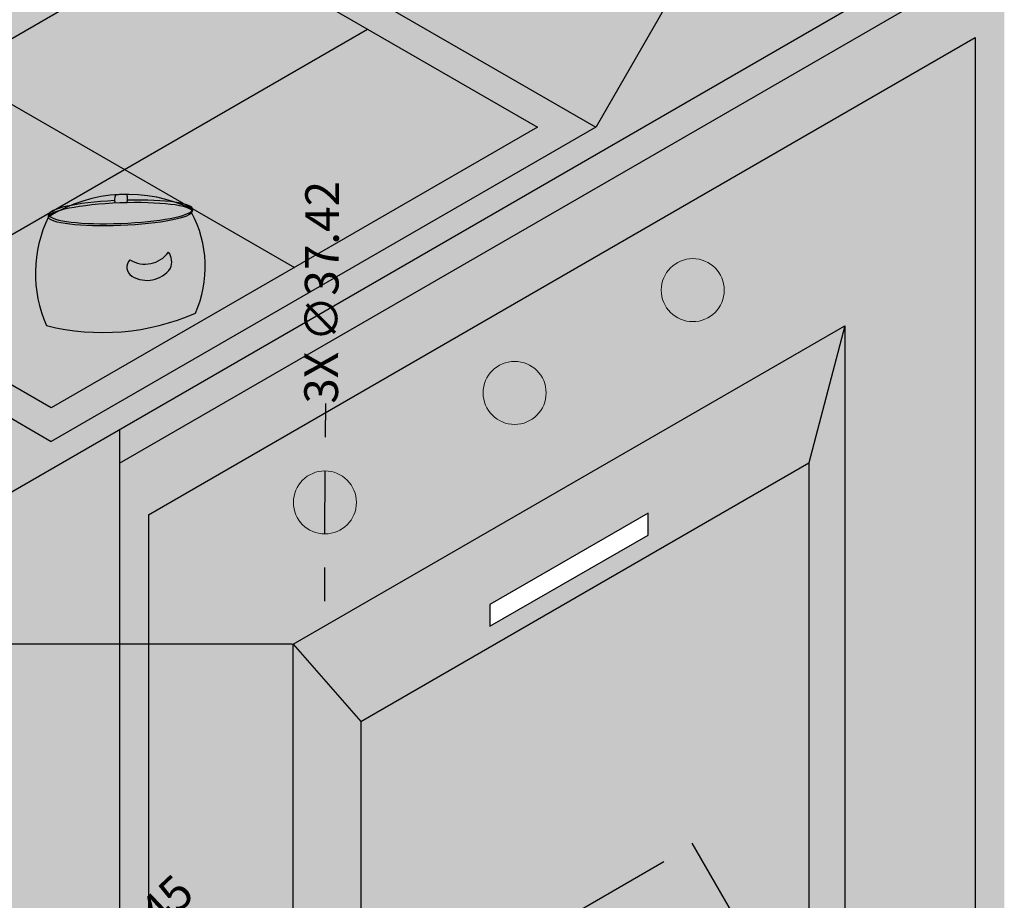
# Model space of a CAD drawing. Units: millimetres. Extents: x 78378 to 86415, y 148682 to 152721.
# Tile 4 of 18: x 79199 to 79783, y 149702 to 150225. Entities that reach past the tile are written whole.
import ezdxf

# ---------------------------------------------------------------- set-up
doc = ezdxf.new("R2010")
doc.units = ezdxf.units.MM
for name, color, linetype, lineweight in [('A-ANNO-DIMS', 2, 'Continuous', 18), ('A-EQPM', 8, 'Continuous', 18), ('A-FURN', 4, 'Continuous', 25), ('A-FURN-PATT', 32, 'Continuous', 13)]:
    doc.layers.add(name, color=color, linetype=linetype, lineweight=lineweight)
doc.styles.get("Standard").update_dxf_attribs({"font": 'arial.ttf'})
doc.dimstyles.new('ISO-25', dxfattribs={"dimtxt": 20, "dimasz": 20, "dimexe": 1.25, "dimexo": 0.625, "dimtad": 0, "dimdec": 1, "dimtxsty": 'Standard', "dimcen": 2.5, "dimadec": 0, "dimazin": 0, "dimtfac": 1, "dimtdec": 1, "dimtmove": 0, "dimatfit": 3, "dimfxl": 1, "dimarcsym": 0})

# ---------------------------------------------------------------- blocks, each defined once
blk = doc.blocks.new('*D22')
at = {"layer": 'A-ANNO-DIMS', "color": 0, "lineweight": -2, "transparency": 16777216}
for p, q in [((80086.091702, 149630.5489088773), (79995.77920202748, 149786.9747473883)), ((79979.08369395178, 149775.8922156335), (79864.48965899751, 149709.7313187051)), ((79710.61581902203, 149620.892215774), (79825.2098539763, 149687.0531127024)), ((79782.98281099998, 149455.5489088774), (79692.67031094636, 149611.9747475287))]:
    blk.add_line(p, q, dxfattribs=at)
at = {"layer": 'A-ANNO-DIMS', "color": 0, "transparency": 16777216}
for points in [[(79977.41702728512, 149778.7789669795), (79980.75036061846, 149773.0054642876), (79996.40420202748, 149785.8922156335)], [(79708.94915235537, 149623.7789671199), (79712.28248568872, 149618.005464428), (79693.29531094636, 149610.892215774)]]:
    blk.add_solid(points, dxfattribs=at)
at = {"layer": 'Defpoints', "color": 0, "transparency": 16777216}
for p in [(79996.40420202748, 149785.8922156335), (80086.404202, 149630.007643), (79783.29531099998, 149455.007643)]:
    blk.add_point(p, dxfattribs=at)
at = {"layer": 'A-ANNO-DIMS', "color": 0, "transparency": 16777216, "insert": (79844.84975648689, 149698.3922157038), "char_height": 20, "attachment_point": 5, "rotation": 30.000000000013433}
blk.add_mtext('350', dxfattribs=at)
blk = doc.blocks.new('*D23')
at = {"layer": 'A-ANNO-DIMS', "color": 0, "lineweight": -2, "transparency": 16777216}
for p, q in [((79304.00747499999, 150298.1287658774), (79213.69497521779, 150454.5546040586)), ((79196.9994671421, 150443.4720723039), (79082.3421139537, 150377.2746185759)), ((78908.23707901475, 150276.7550297867), (79022.8944322031, 150342.9524835145)), ((78980.60407099998, 150111.4117228773), (78890.29157093907, 150267.8375615414))]:
    blk.add_line(p, q, dxfattribs=at)
at = {"layer": 'A-ANNO-DIMS', "color": 0, "transparency": 16777216}
for points in [[(79195.33280047544, 150446.3588236498), (79198.66613380876, 150440.5853209579), (79214.31997521779, 150453.4720723039)], [(78906.57041234808, 150279.6417811326), (78909.90374568143, 150273.8682784407), (78890.91657093907, 150266.7550297866)]]:
    blk.add_solid(points, dxfattribs=at)
at = {"layer": 'Defpoints', "color": 0, "transparency": 16777216}
for p in [(79214.31997521779, 150453.4720723039), (79304.31997499999, 150297.5875), (78980.91657099998, 150110.870457)]:
    blk.add_point(p, dxfattribs=at)
at = {"layer": 'A-ANNO-DIMS', "color": 0, "transparency": 16777216, "insert": (79052.61827307842, 150360.1135510452), "char_height": 20, "attachment_point": 5, "rotation": 30.000000000010683}
blk.add_mtext('373.4', dxfattribs=at)
blk = doc.blocks.new('*D24')
at = {"layer": 'A-ANNO-DIMS', "color": 0, "lineweight": -2, "transparency": 16777216}
for p, q in [((79304.632475, 150298.1287658773), (79394.94497480572, 150454.5546040993)), ((79411.64048288143, 150443.4720723446), (79475.9245159218, 150406.3576685641)), ((79613.47955571176, 150326.9402293129), (79549.19552267138, 150364.0546330934)), ((79541.112564, 150161.5969228774), (79631.42506378744, 150318.0227610676))]:
    blk.add_line(p, q, dxfattribs=at)
at = {"layer": 'A-ANNO-DIMS', "color": 0, "transparency": 16777216}
for points in [[(79413.30714954808, 150446.3588236905), (79409.97381621476, 150440.5853209986), (79394.31997480574, 150453.4720723446)], [(79615.14622237843, 150329.8269806589), (79611.81288904509, 150324.053477967), (79630.80006378744, 150316.9402293129)]]:
    blk.add_solid(points, dxfattribs=at)
at = {"layer": 'Defpoints', "color": 0, "transparency": 16777216}
for p in [(79630.80006378744, 150316.9402293129), (79304.319975, 150297.5874999999), (79540.800064, 150161.055657)]:
    blk.add_point(p, dxfattribs=at)
at = {"layer": 'A-ANNO-DIMS', "color": 0, "transparency": 16777216, "insert": (79512.5600192966, 150385.2061508287), "char_height": 20, "attachment_point": 5, "rotation": 329.9999999999819}
blk.add_mtext('273.06', dxfattribs=at)
blk = doc.blocks.new('*D25')
at = {"layer": 'A-ANNO-DIMS', "color": 0, "lineweight": -2, "transparency": 16777216}
for p, q in [((79360.47687400001, 149854.025187), (78389.60974600006, 149854.025187)), ((78390.85974600006, 149834.025187), (78390.85974600006, 149656.6150549639)), ((78390.85974600006, 149409.864882), (78390.85974600006, 149587.2750140362)), ((79360.47687400001, 149389.8648820001), (78389.60974600006, 149389.8648820001))]:
    blk.add_line(p, q, dxfattribs=at)
at = {"layer": 'A-ANNO-DIMS', "color": 0, "transparency": 16777216}
for points in [[(78387.52641266673, 149834.025187), (78394.19307933339, 149834.025187), (78390.85974600006, 149854.025187)], [(78387.52641266673, 149409.864882), (78394.19307933339, 149409.864882), (78390.85974600006, 149389.8648820001)]]:
    blk.add_solid(points, dxfattribs=at)
at = {"layer": 'Defpoints', "color": 0, "transparency": 16777216}
for p in [(78390.85974600006, 149854.025187), (79361.10187400003, 149854.025187), (79361.10187400003, 149389.8648820001)]:
    blk.add_point(p, dxfattribs=at)
at = {"layer": 'A-ANNO-DIMS', "color": 0, "transparency": 16777216, "insert": (78390.85974600009, 149621.9450345), "char_height": 20, "attachment_point": 5, "rotation": 90}
blk.add_mtext('464.2', dxfattribs=at)
blk = doc.blocks.new('*D26')
at = {"layer": 'A-ANNO-DIMS', "color": 0, "lineweight": -2, "transparency": 16777216}
for p, q in [((79688.22665700002, 149579.4521508773), (79597.91415684896, 149735.8779896975)), ((79581.21864877327, 149724.7954579428), (79462.90800546345, 149656.4887761799)), ((79288.42238213368, 149555.7494545808), (79406.73302544343, 149624.0561363437)), ((79360.78937400001, 149390.4061478773), (79270.47687405797, 149546.8319863355))]:
    blk.add_line(p, q, dxfattribs=at)
at = {"layer": 'A-ANNO-DIMS', "color": 0, "transparency": 16777216}
for points in [[(79579.55198210661, 149727.6822092888), (79582.88531543993, 149721.9087065969), (79598.53915684894, 149734.7954579428)], [(79286.755715467, 149558.6362059267), (79290.08904880035, 149552.8627032348), (79271.10187405799, 149545.7494545808)]]:
    blk.add_solid(points, dxfattribs=at)
at = {"layer": 'Defpoints', "color": 0, "transparency": 16777216}
for p in [(79598.53915684894, 149734.7954579428), (79688.53915700002, 149578.910885), (79361.10187400001, 149389.864882)]:
    blk.add_point(p, dxfattribs=at)
at = {"layer": 'A-ANNO-DIMS', "color": 0, "transparency": 16777216, "insert": (79434.82051545347, 149640.2724562618), "char_height": 20, "attachment_point": 5, "rotation": 29.999999999996074}
blk.add_mtext('378.1', dxfattribs=at)
blk = doc.blocks.new('*D59')
at = {"layer": 'A-ANNO-DIMS', "color": 0, "lineweight": -2, "transparency": 16777216}
for p, q in [((79380.2029535221, 149996.9614811403), (79380.10138026105, 149976.9617390701)), ((79379.809765, 149919.542789), (79379.999807, 149956.961997)), ((79379.70819173894, 149899.5430469298), (79379.60661847789, 149879.5433048597))]:
    blk.add_line(p, q, dxfattribs=at)
at = {"layer": 'A-ANNO-DIMS', "color": 0, "transparency": 16777216}
for points in [[(79376.76808991603, 149976.978667947), (79383.43467060608, 149976.9448101933), (79379.999807, 149956.961997)], [(79376.37490139392, 149899.5599758067), (79383.04148208397, 149899.526118053), (79379.809765, 149919.542789)]]:
    blk.add_solid(points, dxfattribs=at)
at = {"layer": 'Defpoints', "color": 0, "transparency": 16777216}
for p in [(79379.999807, 149956.961997), (79379.809765, 149919.542789)]:
    blk.add_point(p, dxfattribs=at)
at = {"layer": 'A-ANNO-DIMS', "color": 0, "transparency": 16777216, "insert": (79380.53863115159, 150063.0562972237), "char_height": 20, "attachment_point": 5, "rotation": 89.70901279061175}
blk.add_mtext('3X ∅37.42', dxfattribs=at)
blk = doc.blocks.new('*D61')
at = {"layer": 'A-ANNO-DIMS', "color": 0, "lineweight": -2, "transparency": 16777216}
for p, q in [((79224.2464527337, 149639.5853473998), (79209.69247736683, 149625.8674101999)), ((79095.11556299998, 149517.8722489999), (79195.13850199994, 149612.1494729999))]:
    blk.add_line(p, q, dxfattribs=at)
at = {"layer": 'A-ANNO-DIMS', "color": 0, "transparency": 16777216}
blk.add_solid([(79207.40615450018, 149628.293072761), (79211.97880023348, 149623.4417476387), (79195.13850199994, 149612.1494729999)], dxfattribs=at)
at = {"layer": 'Defpoints', "color": 0, "transparency": 16777216}
for p in [(79195.13850199994, 149612.1494729999), (79095.11556299998, 149517.8722489999)]:
    blk.add_point(p, dxfattribs=at)
at = {"layer": 'A-ANNO-DIMS', "color": 0, "transparency": 16777216, "insert": (79261.9300554774, 149675.1042542876), "char_height": 20, "attachment_point": 5, "rotation": 43.30618098475788}
blk.add_mtext('R137.45', dxfattribs=at)

msp = doc.modelspace()

# ---------------------------------------------------------------- hatches: boundary and pattern name
at = {"layer": 'A-FURN-PATT'}
h = msp.add_hatch(color=256, dxfattribs=at)
h.dxf.hatch_style = 1
h.paths.add_polyline_path([(80389.81355980314, 150935.1811176149), (80389.51309381555, 151105.0076434962), (80164.3464888316, 151105.0076434962), (79904.53886769625, 150955.0076434962), (79433.58476952511, 150683.1021681411), (79459.41281351625, 150662.3818050495), (79243.9048024148, 150537.9581968276), (79160.4069246431, 150518.167363956), (78839.3276210414, 150320.0076434962), (78579.51999990609, 150470.0076434961), (78570.85974586825, 150475.0076434961), (78570.85974586825, 150465.0076434962), (78570.85974586825, 149885.0076434961)])
h.paths.add_polyline_path([(80086.40420249099, 150460.0076434961), (79826.59658135568, 150610.0076434961), (78570.85974586825, 149885.0076434961), (78830.66736700358, 149735.0076434961)])
h.paths.add_polyline_path([(79540.80006404899, 150161.0556565937), (79217.39666007676, 149974.3386142535), (78980.9165707482, 150110.8704574853), (79304.31997472048, 150297.5874998256)], flags=16)
h.paths.add_polyline_path([(79506.15904789761, 150161.0556565937), (79217.39666007677, 149994.3386142535), (79015.55758689957, 150110.8704574853), (79304.31997472048, 150277.5874998256)], flags=0)
edge = h.paths.add_edge_path(flags=0)
edge.add_arc((79247.8635885932, 150177.154059363), 137.979927152229, 256.0025927560106, 293.5594108656914)
edge.add_arc((79240.76712928673, 150078.260535577), 68.08549769177299, 336.0991039681863, 387.369687653981)
edge.add_ellipse((79258.3073696606, 150109.4851683714), major_axis=(-42.62344506003415, -1.659142297571932), ratio=0.1604284291443649, start_angle=0, end_angle=179.0977278657225, ccw=False)
edge.add_arc((79285.21118690472, 150074.2509041072), 77.20964330046426, 155.1233103751286, 203.6557939001038)
edge = h.paths.add_edge_path(flags=0)
edge.add_ellipse((79258.69578401413, 150110.8297486024), major_axis=(-42.62344506003415, -1.659142297571932), ratio=0.1604284291443649, start_angle=350.6039411592706, end_angle=356.2289762200799)
edge.add_line((79219.16897707367, 150111.8937051806), (79218.32684768032, 150109.4140931549))
edge.add_arc((79262.46751974897, 150032.9602064517), 88.28134413732826, 112.39312291994881, 119.99999999999571, ccw=False)
h.paths.add_polyline_path([(79287.06250338514, 150086.9702731333, -0.247702064009433), (79288.19674658246, 150077.2955427019, -0.3904765126137986), (79265.47309673205, 150072.5437639662, -0.4872615262363024), (79264.07897218876, 150082.3768585209, 0.3956043262328261)], flags=0)
h.paths.add_polyline_path([(80389.51309381556, 150935.0076434961), (79826.59658135568, 150610.0076434961), (80086.40420249099, 150460.0076434961), (80692.6219851401, 150460.0076434961), (80952.42960627541, 150610.0076434961)])
edge = h.paths.add_edge_path(flags=16)
edge.add_ellipse((80392.44658491029, 150825.6009587087), major_axis=(-133.0756756189512, 7.721978101297283), ratio=0.424499569836956, start_angle=0, end_angle=360)
edge = h.paths.add_edge_path(flags=0)
edge.add_spline(control_points=[(80269.35411604258, 150832.7436415815), (80269.29193278665, 150831.6720147667), (80269.35031475963, 150830.592249842), (80269.73411879689, 150828.3360718096), (80270.06118209881, 150827.1586823489), (80271.04613754865, 150824.6748448987), (80271.70517726007, 150823.3691586005), (80273.40612032128, 150820.6503360826), (80274.44810410585, 150819.2381263036), (80276.93657810257, 150816.3508564802), (80278.3827638828, 150814.8762414973), (80282.58575216534, 150811.0913237019), (80285.62609899955, 150808.7701423959), (80292.60313446997, 150804.2267034199), (80296.53882829295, 150802.0041234762), (80305.19495220963, 150797.7581273222), (80309.91505114386, 150795.7343743789), (80320.0111596611, 150791.9599857595), (80325.38703862559, 150790.2091628441), (80339.21624322617, 150786.3149836253), (80347.95776464436, 150784.3563224224), (80366.06785395242, 150781.2568288573), (80375.43585590576, 150780.1158444778), (80394.309330179, 150778.7158311894), (80403.81420373028, 150778.4568170495), (80422.465596717, 150778.8319300563), (80431.61154730739, 150779.4662025667), (80449.06079653747, 150781.5837654722), (80457.36359407243, 150783.0675039467), (80472.6698529301, 150786.7766095128), (80479.67258750588, 150789.0032721294), (80490.18936031369, 150793.2813222805), (80494.12675567923, 150795.1967122277), (80501.0145611878, 150799.188512515), (80503.9631522054, 150801.2651387212), (80508.20659370373, 150804.9015163823), (80509.7300059309, 150806.4609393726), (80512.19955536906, 150809.4942049083), (80513.14558327098, 150810.9657349426), (80514.42909982229, 150813.5430698013), (80514.84355071915, 150814.6688389962), (80515.39838138374, 150816.8624682529), (80515.5404646545, 150817.9315158847), (80515.58008082317, 150820.0980035506), (80515.47732053277, 150821.197772811), (80514.99049560675, 150823.5061778107), (80514.6046629432, 150824.7154201442), (80513.48543938114, 150827.2641302181), (80512.7510921682, 150828.6026612985), (80510.88722780815, 150831.3808578872), (80509.75776214547, 150832.8196480674), (80507.0873051963, 150835.7513330261), (80505.5466409065, 150837.243857375), (80501.06238832264, 150841.0944478958), (80497.8199298022, 150843.4575549534), (80490.4173793454, 150848.0619874995), (80486.25822277585, 150850.3037143823), (80477.14480578042, 150854.5642972019), (80472.19085006021, 150856.583496544), (80461.6274878137, 150860.3244857693), (80456.01820904585, 150862.0464562905), (80441.73317330678, 150865.8126742317), (80432.78853232553, 150867.6675482482), (80414.33909310326, 150870.5316780972), (80404.8348928345, 150871.5410542788), (80385.7706775062, 150872.6572210053), (80376.21128671143, 150872.7639759942), (80357.54439280283, 150872.0728395342), (80348.43747055416, 150871.27476178), (80331.16822413795, 150868.8299635098), (80323.00642023917, 150867.1826714935), (80309.47200145545, 150863.5363064667), (80303.8627990537, 150861.6592748057), (80293.8018064812, 150857.5400855607), (80289.35122989668, 150855.2968623192), (80282.77569843757, 150851.2345481044), (80280.34726566746, 150849.4578867352), (80276.26060564672, 150845.9127204516), (80274.60404284154, 150844.1457946164), (80272.31573199967, 150841.1242619346), (80271.53575166185, 150839.8453762844), (80270.34961441216, 150837.3878672019), (80269.94168426798, 150836.2101260174), (80269.5065140611, 150834.2814629481), (80269.3988329965, 150833.5142652193), (80269.35411604258, 150832.7436415815)], knot_values=[0, 0, 0, 0, 0.0975004598125087, 0.0975004598125087, 0.1950009196250173, 0.1950009196250173, 0.2925013794375259, 0.2925013794375259, 0.3900018392500346, 0.3900018392500346, 0.4875022990625432, 0.4875022990625432, 0.6388032241337034, 0.6388032241337034, 0.7901041492048636, 0.7901041492048636, 0.9414050742760238, 0.9414050742760238, 1.092705999347184, 1.092705999347184, 1.312817101002443, 1.312817101002443, 1.532928202657702, 1.532928202657702, 1.753039304312961, 1.753039304312961, 1.973150405968221, 1.973150405968221, 2.19326150762348, 2.19326150762348, 2.413372609278739, 2.413372609278739, 2.569860632934037, 2.569860632934037, 2.726348656589336, 2.726348656589336, 2.844186581547077, 2.844186581547077, 2.962024506504818, 2.962024506504818, 3.060233875946405, 3.060233875946405, 3.158443245387991, 3.158443245387991, 3.256652614829578, 3.256652614829578, 3.354861984271164, 3.354861984271164, 3.453071353712751, 3.453071353712751, 3.551280723154337, 3.551280723154337, 3.649490092595923, 3.649490092595923, 3.803927730406353, 3.803927730406353, 3.958365368216782, 3.958365368216782, 4.112803006027212, 4.112803006027212, 4.267240643837642, 4.267240643837642, 4.489203494974081, 4.489203494974081, 4.711166346110521, 4.711166346110521, 4.93312919724696, 4.93312919724696, 5.155092048383399, 5.155092048383399, 5.377054899519838, 5.377054899519838, 5.557853608626545, 5.557853608626545, 5.738652317733252, 5.738652317733252, 5.872395555677483, 5.872395555677483, 6.006138793621714, 6.006138793621714, 6.109604996023907, 6.109604996023907, 6.2130711984261, 6.2130711984261, 6.283185307179586, 6.283185307179586, 6.283185307179586, 6.283185307179586], degree=3, periodic=0)
edge = h.paths.add_edge_path(flags=0)
edge.add_ellipse((80392.446576265, 150825.6009639553), major_axis=(-101.8397670786795, 3.392257208815831), ratio=0.403492477068114, start_angle=0, end_angle=360)
edge = h.paths.add_edge_path(flags=0)
edge.add_ellipse((80391.1657165424, 150858.3745518381), major_axis=(9.088237780547283, -0.67334552975693), ratio=0.3513541290445306, start_angle=0, end_angle=360)
h.paths.add_polyline_path([(80952.42960627541, 150610.0076434961), (80692.62198514014, 150460.0076434962), (81361.23421645904, 150073.9841917607), (81649.96279182703, 150052.7286159431), (81766.49348583283, 150120.0076434961), (81766.49348583283, 150140.0076434961), (81564.90245463562, 150256.396279624), (81564.88840704803, 150096.1962601479), (81538.90760017018, 150111.1962859926), (81538.92165266915, 150271.3963026331)])
h.paths.add_polyline_path([(81539.035680894, 151571.3304684069), (80867.77935513339, 151958.88048878), (80867.77935513337, 151618.8804887802), (81498.02561065964, 151255.0076434964), (81498.02561065964, 150905.0076434961), (81238.21798952435, 150755.0076434961), (81538.94884401507, 150581.3806037023)])
h.paths.add_polyline_path([(81766.49348583283, 151440.0076434962), (81565.01644300755, 151556.3304684069), (81564.92963647815, 150566.38058618), (81766.49348583283, 150450.0076434962)])
edge = h.paths.add_edge_path()
edge.add_line((81564.92963647815, 150566.38058618), (81564.9136990684, 150384.628856009))
edge.add_ellipse((81552.13037602534, 150358.5718270642), major_axis=(52.62721254190076, 3.506026927036754), ratio=0.4958990548584225, start_angle=367.51697565131457, end_angle=420.0564685523974, ccw=False)
edge.add_ellipse((81552.13037602534, 150358.5718270642), major_axis=(52.62721254190076, 3.506026927036754), ratio=0.4958990548584225, start_angle=351.72974196033346, end_angle=367.51697565131457, ccw=False)
edge.add_ellipse((81552.13037602534, 150345.5015529042), major_axis=(52.62721254190076, 3.506026927036754), ratio=0.4958990548584225, start_angle=352.51169489415116, end_angle=366.30060915387577, ccw=False)
edge.add_line((81603.4463374456, 150342.2038825707), (81603.50642755294, 150340.4474978293))
edge.add_ellipse((81552.13037602534, 150332.1280359686), major_axis=(52.62721254190076, 3.506026927036754), ratio=0.4958990548584225, start_angle=353.6729654395227, end_angle=365.38679972494066, ccw=False)
edge.add_ellipse((81552.13037602534, 150332.1280359686), major_axis=(52.62721254190076, 3.506026927036754), ratio=0.4958990548584225, start_angle=350.9388331002564, end_angle=353.6729654395227)
edge.add_line((81603.86882368504, 150329.8549549892), (81604.0441546891, 150324.7301729966))
edge.add_ellipse((81552.13037602534, 150317.7418284518), major_axis=(52.62721254190076, 3.506026927036754), ratio=0.4958990548584225, start_angle=355.21767463173103, end_angle=363.85533637812415, ccw=False)
edge.add_ellipse((81552.13037602534, 150317.7418284518), major_axis=(52.62721254190076, 3.506026927036754), ratio=0.4958990548584225, start_angle=341.3250873036158, end_angle=355.21767463173103, ccw=False)
edge.add_ellipse((81552.13037602534, 150317.7418284518), major_axis=(52.62721254190076, 3.506026927036754), ratio=0.4958990548584225, start_angle=293.4661701367695, end_angle=341.3250873036158, ccw=False)
edge.add_line((81564.90566138821, 150292.9663898651), (81564.90245463562, 150256.396279624))
edge.add_line((81564.90245463562, 150256.396279624), (81766.49348583283, 150140.0076434961))
edge.add_line((81766.49348583283, 150140.0076434961), (81766.49348583283, 150450.0076434962))
edge.add_line((81766.49348583283, 150450.0076434962), (81564.92963647815, 150566.38058618))
h.paths.add_polyline_path([(81525.57129610774, 150321.5980043728), (81526.59848255829, 150321.3069082928), (81528.6771290606, 150320.947049251)])
h.paths.add_polyline_path([(81512.79027333307, 150326.1128631878), (81514.50580755486, 150325.38873887), (81512.53799543541, 150326.2678422534)])
h.paths.add_polyline_path([(81533.21477271736, 150320.1614841748), (81534.69519629495, 150319.9051905676), (81536.59953044976, 150319.755668921)])
h.paths.add_polyline_path([(81518.62200466282, 150323.6512984944), (81519.22704244989, 150323.3959129888), (81521.28902816366, 150322.8115634216)])
h.paths.add_polyline_path([(81501.21834684846, 150336.259909523), (81500.35429342867, 150338.133928838), (81499.78149159584, 150340.0493926212), (81499.50316348342, 150341.9955259773), (81499.50316348343, 150343.7256661642), (81499.75838934928, 150345.5905095656), (81500.27655404429, 150347.4549063508), (81501.05505607055, 150349.3094961287), (81501.09670215519, 150349.3936770376), (81501.13888119749, 150349.4778172982), (81500.99777251929, 150349.749637304), (81500.86282558287, 150350.0225204294), (81499.50316348342, 150355.0658001372), (81499.95910976747, 150359.5002298216), (81501.89819062682, 150363.9082666975), (81505.26528150582, 150368.1645982632), (81509.96466211145, 150372.148224724), (81515.86273756725, 150375.7458987972), (81522.79183627458, 150378.8553451273), (81530.55497651099, 150381.3881677888), (81538.93146626501, 150383.2723632221), (81538.94884401507, 150581.3806037023), (80632.00020687521, 151105.0076434962), (80389.51309381555, 151105.0076434962), (80389.81417426979, 150934.8338146148), (80952.42960627541, 150610.0076434961), (81538.92165266915, 150271.3963026331), (81538.92343538092, 150291.719410528), (81538.87516273293, 150291.7210326448), (81530.1914951021, 150292.8238998863), (81522.18015347481, 150294.6903872688), (81515.08664870211, 150297.2632955209), (81509.86347084012, 150299.9959433281), (81505.6084410237, 150303.1350709547), (81502.41902318504, 150306.608774857), (81500.3682727948, 150310.3374878268), (81499.50316348343, 150314.2358015248), (81499.50316348343, 150315.9659417118), (81499.82059494797, 150318.1159244827), (81500.4869945128, 150320.2634115907), (81501.49791650465, 150322.3940767571), (81500.48699451279, 150324.4232810552), (81499.82059494796, 150326.50388518), (81499.50316348343, 150328.6220090417), (81499.50316348343, 150330.3521492286), (81499.78149159584, 150332.3262168982), (81500.35429342862, 150334.2991697576)])
h = msp.add_hatch(color=256, dxfattribs=at)
h.dxf.hatch_style = 1
h.paths.add_polyline_path([(79783.29531116647, 150265.0076434962), (79783.29531116647, 150285.0076434962), (79257.85559544402, 149981.6448821809), (79257.85559544402, 149961.6448821809)])
h.paths.add_polyline_path([(80086.40420249102, 150440.0076434961), (80086.40420249102, 150460.0076434962), (79783.29531116647, 150285.0076434962), (79783.29531116647, 150265.0076434962)])
h = msp.add_hatch(color=256, dxfattribs=at)
h.dxf.hatch_style = 1
h.paths.add_polyline_path([(79304.31997472048, 150297.5874998256), (78980.9165707482, 150110.8704574853), (79217.39666007676, 149974.3386142535), (79540.80006404899, 150161.0556565937)])
h.paths.add_polyline_path([(79506.1590478976, 150161.0556565937), (79217.39666007677, 149994.3386142535), (79015.55758689957, 150110.8704574853), (79304.31997472048, 150277.5874998256)], flags=16)
edge = h.paths.add_edge_path(flags=0)
edge.add_line((79260.85831739863, 150135.9630570396), (79296.36602525097, 150115.4626723527))
edge.add_ellipse((79258.69578401413, 150110.8297486024), major_axis=(-42.62344506003415, -1.659142297571932), ratio=0.1604284291443649, start_angle=540.162499654083, end_angle=544.7822410835257, ccw=False)
edge.add_ellipse((79258.69578401413, 150110.8297486024), major_axis=(-42.62344506003415, -1.659142297571932), ratio=0.1604284291443649, start_angle=539.9999999999861, end_angle=540.162499654083, ccw=False)
edge.add_line((79301.31133672483, 150112.607495442), (79301.41168660196, 150112.5495584135))
edge.add_ellipse((79258.69578401413, 150110.8297486024), major_axis=(-42.62344506003415, -1.659142297571932), ratio=0.1604284291443649, start_angle=538.6064400413018, end_angle=539.6688473425907, ccw=False)
edge.add_arc((79299.13775409514, 150112.0106508173), 2.233281590130633, -43.6788662491187, 8.993750311263227, ccw=False)
edge.add_arc((79240.76712928673, 150078.260535577), 68.08549769177301, -23.900896031813716, 28.232395801308996, ccw=False)
edge.add_arc((79247.8635885932, 150177.154059363), 137.9799271522289, 256.0025927560107, 293.55941086569135, ccw=False)
edge.add_arc((79285.21118690472, 150074.2509041072), 77.20964330046431, 154.2238313632793, 203.6557939001039, ccw=False)
edge.add_ellipse((79258.3073696606, 150109.4851683714), major_axis=(-42.62344506003415, -1.659142297571932), ratio=0.1604284291443649, start_angle=359.9882644796014, end_angle=360, ccw=False)
edge.add_arc((79216.84611586262, 150108.3941298374), 1.290075563935423, 125.5884183457598, 205.6940851275714, ccw=False)
edge.add_ellipse((79258.69578401413, 150110.8297486024), major_axis=(-42.62344506003415, -1.659142297571932), ratio=0.1604284291443649, start_angle=358.12188373566687, end_angle=359.6349870137668, ccw=False)
edge.add_line((79216.51003741624, 150110.3585656536), (79216.88243710011, 150110.5735707114))
edge.add_ellipse((79258.69578401413, 150110.8297486024), major_axis=(-42.62344506003415, -1.659142297571932), ratio=0.1604284291443649, start_angle=356.2289762200799, end_angle=358.12188373566687, ccw=False)
edge.add_line((79219.16897707361, 150111.8937051806), (79260.85831739863, 150135.9630570396))
h.paths.add_polyline_path([(79288.19674658247, 150077.2955427019, -0.3904765126100298), (79265.47309673225, 150072.5437639661, -0.4872615262481483), (79264.07897218876, 150082.3768585209, 0.3956043262329599), (79287.06250338514, 150086.9702731333, -0.2477020640089524)], flags=0)
h = msp.add_hatch(color=256, dxfattribs=at)
h.dxf.hatch_style = 1
edge = h.paths.add_edge_path()
edge.add_line((79506.15904789761, 150161.0556565937), (79405.23951130905, 150219.3215782097))
edge.add_line((79405.23951130905, 150219.3215782097), (79260.85831739863, 150135.9630570396))
edge.add_line((79260.85831739863, 150135.9630570396), (79296.36602525097, 150115.4626723527))
edge.add_ellipse((79258.69578401413, 150110.8297486024), major_axis=(-42.62344506003415, -1.659142297571932), ratio=0.1604284291443649, start_angle=540.162499654083, end_angle=544.7822410835257, ccw=False)
edge.add_ellipse((79258.69578401413, 150110.8297486024), major_axis=(-42.62344506003415, -1.659142297571932), ratio=0.1604284291443649, start_angle=538.6064400413018, end_angle=539.6688473425907, ccw=False)
edge.add_line((79301.41168660196, 150112.5495584135), (79361.7778539872, 150077.6971354236))
edge.add_line((79361.7778539872, 150077.6971354236), (79506.15904789761, 150161.0556565937))
h.paths.add_polyline_path([(79405.23951130905, 150219.3215782097), (79304.31997472048, 150277.5874998256), (79159.93878081007, 150194.2289786555), (79260.85831739861, 150135.9630570396)])
edge = h.paths.add_edge_path()
edge.add_line((79260.85831739863, 150135.9630570396), (79159.93878081007, 150194.2289786555))
edge.add_line((79159.93878081007, 150194.2289786555), (79015.55758689957, 150110.8704574853))
edge.add_line((79015.55758689957, 150110.8704574853), (79116.47712348816, 150052.6045358695))
edge.add_line((79116.47712348816, 150052.6045358695), (79216.88243710011, 150110.5735707114))
edge.add_ellipse((79258.69578401413, 150110.8297486024), major_axis=(-42.62344506003415, -1.659142297571932), ratio=0.1604284291443649, start_angle=356.2289762200799, end_angle=358.12188373566687, ccw=False)
edge.add_ellipse((79258.69578401413, 150110.8297486024), major_axis=(-42.62344506003415, -1.659142297571932), ratio=0.1604284291443649, start_angle=350.6039411592706, end_angle=356.2289762200799)
edge.add_line((79219.16897707367, 150111.8937051806), (79260.85831739863, 150135.9630570396))
h.paths.add_polyline_path([(79300.75291231953, 150110.4683114996, 0.2164222898616657), (79301.36195664505, 150112.211821585, 0.2592774297089186), (79215.68392460057, 150107.8260260738, 0.2190957382297344), (79214.4892815114, 150043.2712153398, 0.1653553521393526), (79303.0141334557, 150050.6752955396, 0.2314808679006391)], flags=16)
h.paths.add_polyline_path([(79264.07897218876, 150082.3768585209, 0.3956043262329531), (79287.06250338514, 150086.9702731333, -0.2477020640089404), (79288.19674658247, 150077.2955427019, -0.3904765126101912), (79265.47309673225, 150072.5437639661, -0.4872615262477145)], flags=0)
h.paths.add_polyline_path([(79361.7778539872, 150077.6971354236), (79301.41168660196, 150112.5495584135), (79260.85831739863, 150135.9630570395), (79116.47712348816, 150052.6045358695), (79217.39666007677, 149994.3386142535)])
edge = h.paths.add_edge_path(flags=16)
edge.add_ellipse((79258.3073696606, 150109.4851683714), major_axis=(-42.62344506003415, -1.659142297571932), ratio=0.1604284291443649, start_angle=180.4067093272145, end_angle=238.20589381526509, ccw=False)
edge.add_arc((79299.13775409514, 150112.0106508173), 2.233281590130633, 335.7071143626492, 365.1681260371621)
edge.add_arc((79262.46751974897, 150032.9602064517), 88.28134413732828, 63.85950992659765, 90.1998686299514)
edge.add_arc((79256.96489807896, 150118.7368489296), 5.76674788420442, -23.322009605085498, 25.737075277592908, ccw=False)
edge = h.paths.add_edge_path(flags=0)
edge.add_ellipse((79258.3073696606, 150109.4851683714), major_axis=(-42.62344506003415, -1.659142297571932), ratio=0.1604284291443649, start_angle=0, end_angle=179.0977278657225, ccw=False)
edge.add_arc((79285.21118690472, 150074.2509041072), 77.20964330046367, 154.2238313632793, 203.6557939001038)
edge.add_arc((79247.8635885932, 150177.154059363), 137.9799271522199, 256.0025927560106, 293.5594108656914)
edge.add_arc((79240.76712928675, 150078.260535577), 68.08549769176636, 336.0991039681814, 388.2323958012816)
h = msp.add_hatch(color=256, dxfattribs=at)
h.dxf.hatch_style = 1
h.paths.add_polyline_path([(79765.97480309078, 150214.3023755343), (79275.17610351971, 149930.939614219), (79275.17610351968, 149340.2556153015), (79361.10187436163, 149389.8648822274), (79361.10187436163, 149854.0251874417), (79688.53915659874, 150043.071190484), (79688.53915659874, 149578.9108852697), (79765.97480309078, 149623.6183766168)], flags=0)
h.paths.add_polyline_path([(79616.99747211508, 150064.3357852431, -1), (79579.57778226466, 150064.3357852431, -1)], flags=0)
h.paths.add_polyline_path([(79511.25702160504, 150003.2865076769, -1), (79473.83733175462, 150003.2865076769, -1)], flags=0)
h.paths.add_polyline_path([(79398.61463104078, 149938.2523931624, -1), (79361.19494119036, 149938.2523931624, -1)], flags=0)
h.paths.add_polyline_path([(79688.53915659874, 149578.9108852697), (79667.16069404285, 149674.8368362752), (79401.25237372774, 149521.3145959615), (79361.10187436163, 149389.8648822274)], flags=0)
h.paths.add_polyline_path([(79783.29531116645, 149613.6183766167), (79783.29531116647, 150126.6366131478), (79783.29531116647, 150265.0076434962), (79257.85559544402, 149961.6448821809), (79257.85559544401, 149310.2556153015)])
h.paths.add_polyline_path([(79275.17610351968, 149340.2556153015), (79275.17610351971, 149930.939614219), (79765.97480309078, 150214.3023755343), (79765.97480309078, 149623.6183766168)], flags=16)
h.paths.add_polyline_path([(79361.10187436163, 149389.8648822274), (79361.10187436163, 149854.0251874417), (79688.53915659874, 150043.071190484), (79688.53915659874, 149578.9108852697), (79667.16069404285, 149674.8368362752), (79401.25237372774, 149521.3145959615)], flags=0)
h.paths.add_polyline_path([(79477.90289169294, 149864.6773096294), (79477.90289169294, 149877.6075739832), (79571.78517238796, 149931.8105340146), (79571.78517238796, 149918.8802696608)], flags=0)
h = msp.add_hatch(color=256, dxfattribs=at)
h.dxf.hatch_style = 1
h.set_gradient(color1=(39, 118, 187), color2=(122, 175, 223))
h.paths.add_polyline_path([(79667.16069404285, 149961.6902649834), (79401.25237372774, 149808.1680246697), (79401.25237372774, 149521.3145959615), (79667.16069404285, 149674.8368362752)], flags=17)
h.paths.add_polyline_path([(79765.97480309078, 150214.3023755343), (79275.17610351971, 149930.939614219), (79275.17610351968, 149340.2556153015), (79361.10187436163, 149389.8648822274), (79361.10187436163, 149854.0251874417), (79688.53915659874, 150043.071190484), (79688.53915659874, 149578.9108852697), (79765.97480309078, 149623.6183766168)])
h.paths.add_polyline_path([(79579.57778226466, 150064.3357852431, -1), (79616.99747211508, 150064.3357852431, -1)], flags=16)
h.paths.add_polyline_path([(79511.25702160504, 150003.2865076769, -1), (79473.83733175462, 150003.2865076769, -1)], flags=16)
h.paths.add_polyline_path([(79398.61463104078, 149938.2523931624, -1), (79361.19494119036, 149938.2523931624, -1)], flags=16)
h = msp.add_hatch(color=256, dxfattribs=at)
h.dxf.hatch_style = 1
h.paths.add_polyline_path([(79288.19674658247, 150077.2955427019, 0.2477020640089395), (79287.06250338514, 150086.9702731333, -0.3956043262329522), (79264.07897218876, 150082.3768585209, 0.4724153799249179), (79265.21321538703, 150072.702128089, 0.3956043262140555)])
edge = h.paths.add_edge_path()
edge.add_ellipse((79258.3073696606, 150109.4851683714), major_axis=(-42.62344506003415, -1.659142297571932), ratio=0.1604284291443649, start_angle=0, end_angle=179.0977278657224)
edge.add_ellipse((79258.3073696606, 150109.4851683714), major_axis=(-42.62344506003415, -1.659142297571932), ratio=0.1604284291443649, start_angle=179.0977278657224, end_angle=180.4067093272144)
edge.add_ellipse((79258.69578401413, 150110.8297486024), major_axis=(-42.62344506003415, -1.659142297571932), ratio=0.1604284291443649, start_angle=361.19113022594513, end_angle=538.6064400413018, ccw=False)
edge.add_arc((79262.46751974897, 150032.9602064517), 88.28134413732829, 121.4091328036964, 122.0012323120865)
edge = h.paths.add_edge_path()
edge.add_ellipse((79258.3073696606, 150109.4851683714), major_axis=(-42.62344506003415, -1.659142297571932), ratio=0.1604284291443649, start_angle=180.4067093272145, end_angle=353.5884042062345, ccw=False)
edge.add_ellipse((79258.69578401413, 150110.8297486024), major_axis=(-42.62344506003415, -1.659142297571932), ratio=0.1604284291443649, start_angle=538.6064400413017, end_angle=539.6688473425907)
edge.add_arc((79262.46751974897, 150032.9602064517), 88.28134413732826, 63.90344247420405, 116.3789074587053)
edge = h.paths.add_edge_path()
edge.add_ellipse((79258.69578401413, 150110.8297486024), major_axis=(-42.62344506003415, -1.659142297571932), ratio=0.1604284291443649, start_angle=350.6039411592706, end_angle=356.2289762200799)
edge.add_line((79219.16897707366, 150111.8937051806), (79216.88243710002, 150110.5735707113))
edge.add_ellipse((79258.69578401413, 150110.8297486024), major_axis=(-42.62344506003415, -1.659142297571932), ratio=0.1604284291443649, start_angle=358.1218837356668, end_angle=360.4067093272139)
edge.add_ellipse((79258.3073696606, 150109.4851683714), major_axis=(-42.62344506003415, -1.659142297571932), ratio=0.1604284291443649, start_angle=353.5884042062345, end_angle=358.6064400413013, ccw=False)
edge.add_arc((79262.46751974897, 150032.9602064517), 88.28134413732826, 112.39312291993289, 116.37890745869689, ccw=False)
edge = h.paths.add_edge_path(flags=17)
edge.add_ellipse((79258.69578401413, 150110.8297486024), major_axis=(-42.62344506003415, -1.659142297571932), ratio=0.1604284291443649, start_angle=180.162499654083, end_angle=184.7822410835257)
edge.add_line((79296.36602525097, 150115.4626723527), (79301.30786510574, 150112.6094997823))
edge = h.paths.add_edge_path()
edge.add_ellipse((79258.69578401413, 150110.8297486024), major_axis=(-42.62344506003415, -1.659142297571932), ratio=0.1604284291443649, start_angle=539.6688473425907, end_angle=539.9999999999861, ccw=False)
edge.add_ellipse((79258.69578401413, 150110.8297486024), major_axis=(-42.62344506003415, -1.659142297571932), ratio=0.1604284291443649, start_angle=538.6064400413018, end_angle=539.6688473425907, ccw=False)
edge.add_ellipse((79258.3073696606, 150109.4851683714), major_axis=(-42.62344506003415, -1.659142297571932), ratio=0.1604284291443649, start_angle=179.0977278657225, end_angle=180.4067093272145, ccw=False)
edge.add_arc((79299.13775409514, 150112.0106508173), 2.233281590130633, 316.3211337490277, 372.3652135005989)
edge = h.paths.add_edge_path()
edge.add_line((79301.30786510574, 150112.6094997823), (79296.36602525094, 150115.4626723527))
edge.add_ellipse((79258.69578401413, 150110.8297486024), major_axis=(-42.62344506003415, -1.659142297571932), ratio=0.1604284291443649, start_angle=184.7822410835257, end_angle=187.8201250283657)
edge.add_arc((79262.46751974897, 150032.9602064517), 88.28134413732823, 63.903442474203985, 71.2108858215264, ccw=False)
edge.add_ellipse((79258.69578401413, 150110.8297486024), major_axis=(-42.62344506003415, -1.659142297571932), ratio=0.1604284291443649, start_angle=539.6688473425907, end_angle=539.9999999999861)
edge.add_ellipse((79258.69578401413, 150110.8297486024), major_axis=(-42.62344506003415, -1.659142297571932), ratio=0.1604284291443649, start_angle=539.9999999999861, end_angle=180.162499654083)
h = msp.add_hatch(color=256, dxfattribs=at)
h.dxf.hatch_style = 1
edge = h.paths.add_edge_path()
edge.add_ellipse((79258.3073696606, 150109.4851683714), major_axis=(-42.62344506003415, -1.659142297571932), ratio=0.1604284291443649, start_angle=0, end_angle=179.0977278657225, ccw=False)
edge.add_arc((79285.21118690472, 150074.2509041072), 77.20964330046426, 154.2238313632793, 203.6557939001038)
edge.add_arc((79247.8635885932, 150177.154059363), 137.9799271522289, 256.0025927560106, 293.5594108656914)
edge.add_arc((79240.76712928673, 150078.260535577), 68.08549769177301, 336.0991039681863, 388.2323958012758)
h.paths.add_polyline_path([(79264.07897218876, 150082.3768585209, 0.3956043262329519), (79287.06250338514, 150086.9702731333, -0.2477020640089396), (79288.19674658247, 150077.2955427019, -0.3904765126102086), (79265.47309673225, 150072.5437639661, -0.4872615262476615)], flags=0)
edge = h.paths.add_edge_path()
edge.add_ellipse((79258.69578401413, 150110.8297486024), major_axis=(-42.62344506003415, -1.659142297571932), ratio=0.1604284291443649, start_angle=361.1911302259451, end_angle=538.6064400413017)
edge.add_ellipse((79258.3073696606, 150109.4851683714), major_axis=(-42.62344506003415, -1.659142297571932), ratio=0.1604284291443649, start_angle=180.4067093272144, end_angle=238.205893815265)
edge.add_ellipse((79258.3073696606, 150109.4851683714), major_axis=(-42.62344506003415, -1.659142297571932), ratio=0.1604284291443649, start_angle=238.205893815265, end_angle=292.1855356769677)
edge.add_ellipse((79258.3073696606, 150109.4851683714), major_axis=(-42.62344506003415, -1.659142297571932), ratio=0.1604284291443649, start_angle=292.1855356769677, end_angle=353.5884042062345)
edge.add_arc((79262.46751974897, 150032.9602064517), 88.28134413732828, 116.3789074587053, 121.4091328036964)
h.paths.add_polyline_path([(79288.19674658247, 150077.2955427019, 0.2477020640089458), (79287.06250338514, 150086.9702731333, -0.3956043262329522), (79264.07897218876, 150082.3768585209, 0.4724153799249375), (79265.21321538703, 150072.702128089, 0.3956043262140486)], flags=16)
h = msp.add_hatch(color=256, dxfattribs=at)
h.dxf.hatch_style = 1
h.paths.add_polyline_path([(79361.19494119036, 149938.2523931624, 1), (79398.61463104078, 149938.2523931624, 1)])
h.paths.add_polyline_path([(79473.83733175462, 150003.2865076769, 1), (79511.25702160504, 150003.2865076769, 1)])
h.paths.add_polyline_path([(79579.57778226466, 150064.3357852431, 1), (79616.99747211508, 150064.3357852431, 1)])
h = msp.add_hatch(color=256, dxfattribs=at)
h.dxf.hatch_style = 1
h.paths.add_polyline_path([(79401.25237372774, 149808.1680246697), (79361.10187436163, 149854.0251874417), (79361.10187436163, 149389.8648822274), (79401.25237372774, 149521.3145959615)])
h.paths.add_polyline_path([(79667.16069404285, 149961.6902649834), (79688.53915659874, 150043.071190484), (79361.10187436163, 149854.0251874417), (79401.25237372774, 149808.1680246697)])
h.paths.add_polyline_path([(79477.90289169294, 149864.6773096294), (79477.90289169294, 149877.6075739832), (79571.78517238796, 149931.8105340146), (79571.78517238796, 149918.8802696608)], flags=16)
h.paths.add_polyline_path([(79688.53915659874, 150043.071190484), (79667.16069404285, 149961.6902649834), (79667.16069404285, 149674.8368362752), (79688.53915659874, 149578.9108852697)])
h = msp.add_hatch(color=256, dxfattribs=at)
h.dxf.hatch_style = 1
h.paths.add_polyline_path([(78830.66736700358, 149715.0076434961), (78570.85974586825, 149865.0076434961), (78570.85974586825, 149055.0076434961), (78830.66736700357, 148905.0076434961)])
h.paths.add_polyline_path([(79257.85559544402, 149981.6448821809), (78830.66736700358, 149735.0076434961), (78830.66736700357, 148905.0076434961), (79257.85559544401, 149151.6448821809)])
h.paths.add_polyline_path([(79116.9453070066, 149653.5787179994, -0.339994386820015), (79231.87483333048, 149531.6448821809), (79231.87483333048, 149166.6448821809), (78856.6481291171, 148950.0076434961), (78856.64812911711, 149398.1143158829, -0.2534236427703663), (78959.42083981534, 149588.1765595852, -0.7771445345120718)], flags=16)
h.paths.add_polyline_path([(79231.87483333048, 149531.6448821809, 0.3399943868200171), (79116.9453070066, 149653.5787179994, 0.7771445345121064), (78959.42083981536, 149588.1765595852, 0.2534236427703481), (78856.64812911711, 149398.1143158829), (78856.6481291171, 148950.0076434961), (79231.87483333048, 149166.6448821809)], flags=0)

# ---------------------------------------------------------------- linework, layer by layer
at = {"layer": 'A-EQPM'}
for centre in [(79598.28762718987, 150064.3357852431), (79492.54717667983, 150003.2865076769), (79379.90478611557, 149938.2523931624)]:
    msp.add_circle(centre, 18.70984492520802, dxfattribs=at)
at = {"layer": 'A-FURN'}
for p, q in [((78830.66736700358, 149735.0076434961), (80086.40420249102, 150460.0076434962)), ((79257.85559544402, 149961.6448821809), (80086.40420249102, 150440.0076434961)), ((79304.31997472048, 150297.5874998256), (79540.80006404899, 150161.0556565937)), ((79015.5575868996, 150110.8704574854), (79304.31997472052, 150277.5874998256)), ((79304.31997472049, 150277.5874998256), (79506.1590478976, 150161.0556565937)), ((79116.47712348816, 150052.6045358695), (79405.23951130905, 150219.3215782097)), ((79275.17610351971, 149930.939614219), (79765.97480309076, 150214.3023755343)), ((79765.97480309078, 150214.3023755343), (79765.97480309078, 149623.6183766168)), ((79159.93878081006, 150194.2289786555), (79361.7778539872, 150077.6971354236)), ((79540.80006404899, 150161.0556565937), (79217.39666007676, 149974.3386142535)), ((79506.15904789761, 150161.0556565937), (79217.39666007677, 149994.3386142535)), ((79217.40415829117, 149974.3342851574), (78980.9165707482, 150110.8704574853)), ((79217.39666007675, 149994.3386142536), (79015.55758689958, 150110.8704574853)), ((79361.10187436163, 149854.0251874417), (79688.53915659874, 150043.071190484)), ((79688.53915659874, 150043.071190484), (79667.16069404285, 149961.6902649834)), ((79688.53915659874, 150043.071190484), (79688.53915659874, 149578.9108852697)), ((79234.72466636686, 149984.3342851574), (79234.71716815243, 149984.3386142535)), ((79257.85559544402, 149981.6448821809), (79257.85559544401, 149151.6448821809)), ((79401.25237372774, 149808.1680246697), (79667.16069404288, 149961.6902649834)), ((79667.16069404285, 149961.6902649834), (79667.16069404285, 149674.8368362752)), ((79275.17610351971, 149930.939614219), (79275.17610351968, 149340.2556153015)), ((79571.78517238796, 149931.8105340146), (79477.90289169295, 149877.6075739832)), ((79571.78517238796, 149918.8802696608), (79571.78517238796, 149931.8105340146)), ((79477.90289169294, 149864.6773096294), (79571.78517238796, 149918.8802696608)), ((79477.90289169294, 149877.6075739832), (79477.90289169294, 149864.6773096294)), ((79361.10187436163, 149389.8648822274), (79361.10187436163, 149854.0251874417)), ((79361.10187436163, 149854.0251874417), (79401.25237372774, 149808.1680246697)), ((79401.25237372774, 149808.1680246697), (79401.25237372774, 149521.3145959615))]:
    msp.add_line(p, q, dxfattribs=at)
for centre, radius, start, end in [((79262.46751974897, 150032.9602064517), 88.28134413733088, 63.90344247420405, 122.0012323120865), ((79259.59592051107, 150118.1296652185), 4.746556962948185, 147.838530292432, 203.9839627813628), ((79259.41296693134, 150106.8426735204), 14.33613935376209, 78.30853823286697, 105.5169714591858), ((79256.96489807896, 150118.7368489296), 5.766747884198656, 336.6779903949136, 21.83154576480296), ((79299.13775409512, 150112.0106508173), 2.233281590142289, 316.321133751139, 12.36521350051892), ((79285.21118690472, 150074.2509041072), 77.20964330046061, 154.2238313632799, 203.6557939001041), ((79216.84611586262, 150108.3941298374), 1.29007556392567, 125.5884183483153, 205.696015007863), ((79240.76712928672, 150078.260535577), 68.08549769178519, 336.0991039681913, 28.232395801309), ((79268.6232928246, 150078.0057709948), 6.305335534478453, 136.1131601627894, 237.2602432127938), ((79273.12224810582, 150096.924787134), 17.12959620779038, 238.1341105353262, 324.4699737550269), ((79278.46425459838, 150081.0583809234), 10.43457482128232, 338.8621828557865, 34.51122051961156), ((79274.25649130315, 150087.2500567026), 17.12959620779038, 238.1341105353262, 324.4699737550269), ((79247.86358859319, 150177.154059363), 137.9799271522189, 256.0025927560117, 293.5594108656962)]:
    msp.add_arc(centre, radius, start, end, dxfattribs=at)
msp.add_ellipse((79258.69578401413, 150110.8297486024), major_axis=(-42.62344506003415, -1.659142297571932), ratio=0.1604284291443649, start_param=4.795539055480054, end_param=10.89676217842124, dxfattribs=at)
msp.add_ellipse((79258.3073696606, 150109.4851683714), major_axis=(-42.62344506003415, -1.659142297571932), ratio=0.1604284291443649, dxfattribs=at)

# ---------------------------------------------------------------- dimensions: what is measured, and where the dimension line sits
at = {"layer": 'A-ANNO-DIMS'}
for base, p1, p2, angle, override, picture, middle in [((79214.31997521779, 150453.4720723039), (78980.916571, 150110.870457), (79304.319975, 150297.5875), 30.00000000001068, {"dimdec": 1, "dimlfac": 1, "dimrnd": 0, "dimzin": 0, "dimdsep": 46, "dimlunit": 2}, '*D23', (79052.61827307842, 150360.1135510452)), ((79630.80006378744, 150316.9402293129), (79304.319975, 150297.5875), (79540.800064, 150161.055657), 329.9999999999819, {"dimdec": 2, "dimlfac": 1, "dimrnd": 0, "dimzin": 0, "dimdsep": 46, "dimlunit": 2}, '*D24', (79512.5600192966, 150385.2061508287)), ((78390.85974600006, 149854.025187), (79361.101874, 149389.864882), (79361.101874, 149854.025187), 90, {"dimdec": 1, "dimlfac": 1, "dimrnd": 0, "dimzin": 0, "dimdsep": 46, "dimlunit": 2}, '*D25', (78390.85974600009, 149621.9450345)), ((79996.40420202748, 149785.8922156335), (79783.295311, 149455.007643), (80086.404202, 149630.007643), 30.00000000001342, {"dimdec": 0, "dimlfac": 1, "dimrnd": 0, "dimzin": 0, "dimdsep": 46, "dimlunit": 2}, '*D22', (79844.84975648689, 149698.3922157038)), ((79598.53915684894, 149734.7954579428), (79361.101874, 149389.864882), (79688.539157, 149578.910885), 29.99999999999607, {"dimdec": 1, "dimlfac": 1, "dimrnd": 0, "dimzin": 0, "dimdsep": 46, "dimlunit": 2}, '*D26', (79434.82051545347, 149640.2724562618))]:
    dim = msp.add_linear_dim(base=base, p1=p1, p2=p2, angle=angle, dimstyle='ISO-25', override=override, dxfattribs=at)
    dim.commit()
    dim.dimension.update_dxf_attribs({"geometry": picture, "text_midpoint": middle})
dim = msp.add_diameter_dim_2p(p1=(79379.809765, 149919.542789), p2=(79379.999807, 149956.961997), text='3X <>', dimstyle='ISO-25', override={"dimdec": 2, "dimlfac": 1, "dimrnd": 0, "dimzin": 0, "dimdsep": 46, "dimlunit": 2}, dxfattribs=at)
dim.commit()
dim.dimension.update_dxf_attribs({"geometry": '*D59', "text_midpoint": (79380.53863115159, 150063.0562972237), "dimtype": 163})
dim = msp.add_radius_dim(center=(79095.11556299998, 149517.8722489999), mpoint=(79195.13850199994, 149612.1494729999), dimstyle='ISO-25', override={"dimdec": 2, "dimlfac": 1, "dimrnd": 0, "dimzin": 0, "dimdsep": 46, "dimlunit": 2}, dxfattribs=at)
dim.commit()
dim.dimension.update_dxf_attribs({"geometry": '*D61', "text_midpoint": (79261.9300554774, 149675.1042542876)})

doc.saveas('drawing.dxf')
